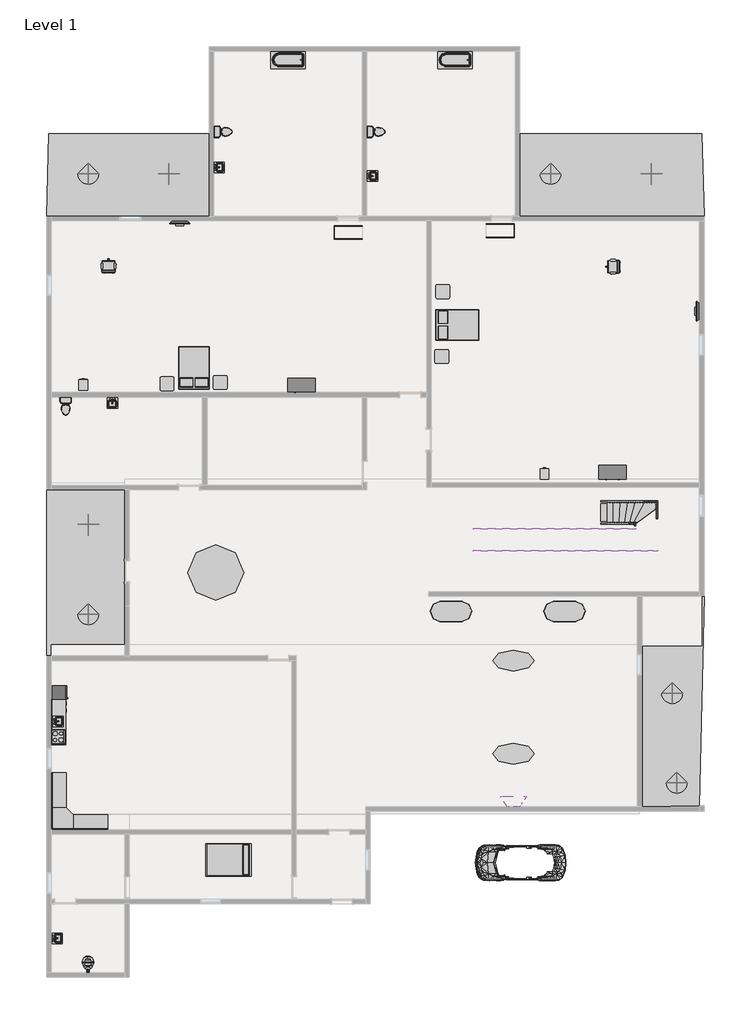
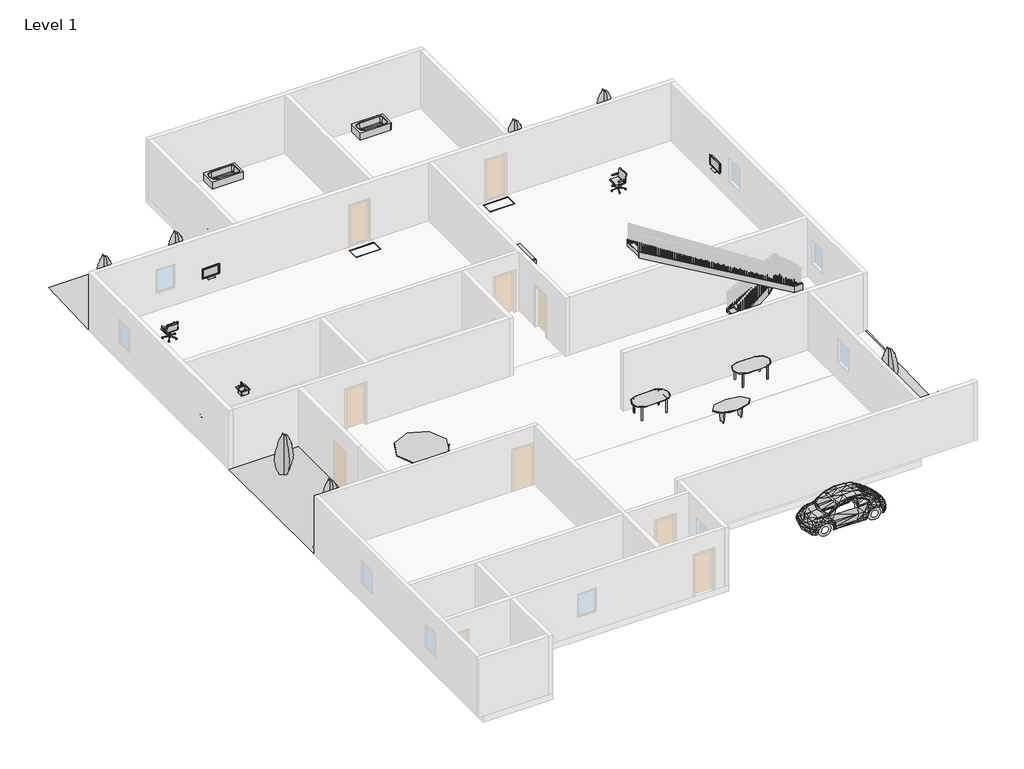
# One storey, part 4 of 4: 23 furniture elements, 11 flow terminals, 11 proxies, 8 geographic elements, 8 members, 1 stair flight.
"""IFC4 building model written with IfcOpenShell, lengths in millimetres."""

from ifc_helpers import new_model, si_unit, frame, origin, place, context, project, spatial, polyline, outline, extrude, triangles, transform, mapped, element, save
from components import proxy_a6faaae8, proxy_45b28599, kitchenette_medium_kitchenette_medium_844211aa, rpc_beetle_rpc_beetle_3ce7ba48, proxy_c523a7b7, walk_off_mat_walk_off_mat_25c2b8c1, flow_terminal_871c2e40, flow_terminal_bd37145e, toilet_domestic_3d_toilet_domestic_3d_f7549cf7, toilet_domestic_3d_toilet_domestic_3d_183bbd19, tub_rectangular_3d_tub_rectangular_3d_ca47631e, furniture_c8abb964, furniture_096e7f55, furniture_552c1472, chair_task_arms_chair_task_arms_fa5a08ef, furniture_c6510c7c, furniture_9fa109b2, furniture_56245f3a, tv_stand_tv_stand_6ce107e5, furniture_2c34a4f9, furniture_5d3b8c6f, furniture_027a2ad9, furniture_bcf351fa, furniture_45e3acac, rpc_tree_conifer_chinese_juniper_7_1b9786cd, stair_flight_225c1673

model = new_model("IFC4")

# Units and contexts
model_context = context("Model", 3, world=origin())
ifc_project = project(units=[si_unit("LENGTHUNIT", "METRE", prefix="MILLI")], contexts=[model_context])

# Site, building, storey
site = spatial("IfcSite", under=ifc_project)
building = spatial("IfcBuilding", under=site)
storey = spatial("IfcBuildingStorey", under=building, Name="Level 1", Elevation=0.0)

# Proxies
placement = place(None, origin())
element("IfcBuildingElementProxy", 1, Name="Building Element Proxy", at=placement, inside=storey, context=model_context, shape_type="Tessellation", body=[
    triangles([(-12619.2832214, 17120.266626, 0.0), (-5481.8828339, 17120.266626, 0.0), (-5583.4830276, 13500.766626, 0.0), (-12720.8828339, 13500.766626, 0.0)], [[1, 4, 3], [3, 2, 1]], closed=False),
])
element("IfcBuildingElementProxy", 2, Name="Building Element Proxy", at=placement, inside=storey, context=model_context, shape_type="Tessellation", body=[
    triangles([(7929.3171661, 17120.266626, 0.0), (16006.5171661, 17120.266626, 0.0), (16108.1167786, 13500.766626, 0.0), (8030.9173599, 13500.766626, 0.0)], [[1, 4, 2], [3, 2, 4]], closed=False),
])
element("IfcBuildingElementProxy", 3, Name="Building Element Proxy", at=placement, inside=storey, context=model_context, shape_type="Tessellation", body=[
    triangles([(-12720.8828339, 1511.9665775, 0.0), (-9291.8828339, 1511.9665775, 0.0), (-9291.8828339, -5777.833374, 0.0), (-12720.8828339, -5777.833374, 0.0)], [[1, 4, 2], [3, 2, 4]], closed=False),
])
element("IfcBuildingElementProxy", 4, Name="Building Element Proxy", at=placement, inside=storey, context=model_context, shape_type="Tessellation", body=[
    triangles([(13390.3175537, -3161.6334709, 0.0), (16108.1167786, -3161.6334709, 0.0), (13390.3175537, -12381.8337616, 0.0), (15904.9175537, -12356.4329865, 0.0)], [[1, 3, 4], [4, 2, 1]], closed=False),
])
proxy_shape = proxy_a6faaae8(model_context)
element("IfcBuildingElementProxy", 5, Name="Cook Top-4 Unit2 : 22\" x 20\"", ObjectType="Cook Top-4 Unit2 : 22\" x 20\"", at=placement, inside=storey, context=model_context, shape_type="MappedRepresentation", body=[
    mapped(proxy_shape, transform((-12212.8828173, -9321.1334604, 0.0), x_axis=(0.0, 1.0, 0.0), y_axis=(-1.0, 0.0, 0.0), z_axis=(0.0, 0.0, 1.0))),
])
proxy_2_shape = proxy_45b28599(model_context)
element("IfcBuildingElementProxy", 6, Name="Dishwasher : 24\" x 24\" x 34\"", ObjectType="Dishwasher : 24\" x 24\" x 34\"", at=placement, inside=storey, context=model_context, shape_type="MappedRepresentation", body=[
    mapped(proxy_2_shape, transform((-11921.0332525, -8369.9509289, 0.0), x_axis=(0.0, 1.0, 0.0), y_axis=(-1.0, 0.0, 0.0), z_axis=(0.0, 0.0, 1.0))),
])
kitchenette_medium_kitchenette_medium_shape = kitchenette_medium_kitchenette_medium_844211aa(model_context)
element("IfcBuildingElementProxy", 7, Name="Kitchenette - Medium : Kitchenette - Medium", ObjectType="Kitchenette - Medium : Kitchenette - Medium", at=placement, inside=storey, context=model_context, shape_type="MappedRepresentation", body=[
    mapped(kitchenette_medium_kitchenette_medium_shape, transform((-12517.6828173, -8996.9711653, 0.0), x_axis=(0.0, 1.0, 0.0), y_axis=(-1.0, 0.0, 0.0), z_axis=(0.0, 0.0, 1.0))),
])
rpc_beetle_rpc_beetle_shape = rpc_beetle_rpc_beetle_3ce7ba48(model_context)
element("IfcBuildingElementProxy", 8, Name="RPC Beetle : RPC Beetle", ObjectType="RPC Beetle : RPC Beetle", at=placement, inside=storey, context=model_context, shape_type="MappedRepresentation", body=[
    mapped(rpc_beetle_rpc_beetle_shape, transform((9300.9171827, -14845.6334604, 0.0), x_axis=(0.0, 1.0, 0.0), y_axis=(-1.0, 0.0, 0.0), z_axis=(0.0, 0.0, 1.0))),
])
proxy_3_shape = proxy_c523a7b7(model_context)
element("IfcBuildingElementProxy", 9, Name="Refrigerator : 24\" x 25\" LH", ObjectType="Refrigerator : 24\" x 25\" LH", at=placement, inside=storey, context=model_context, shape_type="MappedRepresentation", body=[
    mapped(proxy_3_shape, transform((-12167.2338458, -7384.3834604, 0.0), x_axis=(0.0, 1.0, 0.0), y_axis=(-1.0, 0.0, 0.0), z_axis=(0.0, 0.0, 1.0))),
])
walk_off_mat_walk_off_mat_shape = walk_off_mat_walk_off_mat_25c2b8c1(model_context)
element("IfcBuildingElementProxy", 10, Name="Walk-Off Mat : Walk-Off Mat", ObjectType="Walk-Off Mat : Walk-Off Mat", at=placement, inside=storey, context=model_context, shape_type="MappedRepresentation", body=[
    mapped(walk_off_mat_walk_off_mat_shape, transform((905.9526444, 13538.8606067, 0.0), x_axis=(1.0, 0.0, 0.0), y_axis=(0.0, 1.0, 0.0), z_axis=(0.0, 0.0, 1.0))),
])
element("IfcBuildingElementProxy", 11, Name="Walk-Off Mat : Walk-Off Mat", ObjectType="Walk-Off Mat : Walk-Off Mat", at=placement, inside=storey, context=model_context, shape_type="MappedRepresentation", body=[
    mapped(walk_off_mat_walk_off_mat_shape, transform((7560.7526444, 13615.0606067, 0.0), x_axis=(1.0, 0.0, 0.0), y_axis=(0.0, 1.0, 0.0), z_axis=(0.0, 0.0, 1.0))),
])

# Flow terminals
flow_terminal_shape = flow_terminal_871c2e40(model_context)
element("IfcFlowTerminal", 12, ObjectType="Sink Kitchen-Island : 18\" x 18\"", at=placement, inside=storey, context=model_context, shape_type="MappedRepresentation", body=[
    mapped(flow_terminal_shape, transform((-5162.0374161, 15631.3772991, 0.0), x_axis=(0.0, 1.0000000000000002, 0.0), y_axis=(-1.0000000000000002, 0.0, 0.0), z_axis=(0.0, 0.0, 1.0))),
])
element("IfcFlowTerminal", 13, ObjectType="Sink Kitchen-Island : 18\" x 18\"", at=placement, inside=storey, context=model_context, shape_type="MappedRepresentation", body=[
    mapped(flow_terminal_shape, transform((1568.9625839, 15250.3772991, 0.0), x_axis=(0.0, 1.0000000000000009, 0.0), y_axis=(-1.0000000000000009, 0.0, 0.0), z_axis=(0.0, 0.0, 1.0))),
])
element("IfcFlowTerminal", 14, ObjectType="Sink Kitchen-Island : 18\" x 18\"", at=placement, inside=storey, context=model_context, shape_type="MappedRepresentation", body=[
    mapped(flow_terminal_shape, transform((-9853.6720578, 5306.9211385, 0.0), x_axis=(1.0, 0.0, 0.0), y_axis=(0.0, 1.0, 0.0), z_axis=(0.0, 0.0, 1.0))),
])
element("IfcFlowTerminal", 15, ObjectType="Sink Kitchen-Island : 18\" x 18\"", at=placement, inside=storey, context=model_context, shape_type="MappedRepresentation", body=[
    mapped(flow_terminal_shape, transform((-12210.5374161, -8663.7227009, -14.4), x_axis=(0.0, 1.0, 0.0), y_axis=(-1.0, 0.0, 0.0), z_axis=(0.0, 0.0, 1.0))),
])
element("IfcFlowTerminal", 16, ObjectType="Sink Kitchen-Island : 18\" x 18\"", at=placement, inside=storey, context=model_context, shape_type="MappedRepresentation", body=[
    mapped(flow_terminal_shape, transform((-12248.6374161, -18176.0227009, 0.0), x_axis=(0.0, 1.0000000000000002, 0.0), y_axis=(-1.0000000000000002, 0.0, 0.0), z_axis=(0.0, 0.0, 1.0))),
])
flow_terminal_2_shape = flow_terminal_bd37145e(model_context)
element("IfcFlowTerminal", 17, ObjectType="Toilet-Commercial-Wall-3D : 15\" Seat Height", at=placement, inside=storey, context=model_context, shape_type="MappedRepresentation", body=[
    mapped(flow_terminal_2_shape, transform((-11309.6859711, -19773.2334604, 0.0), x_axis=(1.0, 0.0, 0.0), y_axis=(0.0, 1.0, 0.0), z_axis=(0.0, 0.0, 1.0))),
])
toilet_domestic_3d_toilet_domestic_3d_shape = toilet_domestic_3d_toilet_domestic_3d_f7549cf7(model_context)
toilet_domestic_3d_toilet_domestic_3d_2_shape = toilet_domestic_3d_toilet_domestic_3d_183bbd19(model_context)
element("IfcFlowTerminal", 18, ObjectType="Toilet-Domestic-3D : Toilet-Domestic-3D", at=placement, inside=storey, context=model_context, shape_type="MappedRepresentation", body=[
    mapped(toilet_domestic_3d_toilet_domestic_3d_shape, transform((-4885.5867899, 17203.8414884, 0.0), x_axis=(0.0, 1.0000000000000002, 0.0), y_axis=(-1.0000000000000002, 0.0, 0.0), z_axis=(0.0, 0.0, 1.0))),
    mapped(toilet_domestic_3d_toilet_domestic_3d_2_shape, transform((-4885.5867899, 17203.8414884, 0.0), x_axis=(0.0, 1.0000000000000002, 0.0), y_axis=(-1.0000000000000002, 0.0, 0.0), z_axis=(0.0, 0.0, 1.0))),
])
element("IfcFlowTerminal", 19, ObjectType="Toilet-Domestic-3D : Toilet-Domestic-3D", at=placement, inside=storey, context=model_context, shape_type="MappedRepresentation", body=[
    mapped(toilet_domestic_3d_toilet_domestic_3d_shape, transform((1820.0132101, 17203.8414884, 0.0), x_axis=(0.0, 1.0000000000000002, 0.0), y_axis=(-1.0000000000000002, 0.0, 0.0), z_axis=(0.0, 0.0, 1.0))),
    mapped(toilet_domestic_3d_toilet_domestic_3d_2_shape, transform((1820.0132101, 17203.8414884, 0.0), x_axis=(0.0, 1.0000000000000002, 0.0), y_axis=(-1.0000000000000002, 0.0, 0.0), z_axis=(0.0, 0.0, 1.0))),
])
element("IfcFlowTerminal", 20, ObjectType="Toilet-Domestic-3D : Toilet-Domestic-3D", at=placement, inside=storey, context=model_context, shape_type="MappedRepresentation", body=[
    mapped(toilet_domestic_3d_toilet_domestic_3d_shape, transform((-11882.6828173, 5081.2705123, 0.0), x_axis=(1.0, 0.0, 0.0), y_axis=(0.0, 1.0, 0.0), z_axis=(0.0, 0.0, 1.0))),
    mapped(toilet_domestic_3d_toilet_domestic_3d_2_shape, transform((-11882.6828173, 5081.2705123, 0.0), x_axis=(1.0, 0.0, 0.0), y_axis=(0.0, 1.0, 0.0), z_axis=(0.0, 0.0, 1.0))),
])
tub_rectangular_3d_tub_rectangular_3d_shape = tub_rectangular_3d_tub_rectangular_3d_ca47631e(model_context)
element("IfcFlowTerminal", 21, ObjectType="Tub-Rectangular-3D : Tub-Rectangular-3D", at=placement, inside=storey, context=model_context, shape_type="MappedRepresentation", body=[
    mapped(tub_rectangular_3d_tub_rectangular_3d_shape, transform((-2477.685786, 20841.3665396, 0.0), x_axis=(-1.0, 0.0, 0.0), y_axis=(0.0, -1.0, 0.0), z_axis=(0.0, 0.0, 1.0))),
])
element("IfcFlowTerminal", 22, ObjectType="Tub-Rectangular-3D : Tub-Rectangular-3D", at=placement, inside=storey, context=model_context, shape_type="MappedRepresentation", body=[
    mapped(tub_rectangular_3d_tub_rectangular_3d_shape, transform((4837.514214, 20841.3665396, 0.0), x_axis=(-1.0, 0.0, 0.0), y_axis=(0.0, -1.0, 0.0), z_axis=(0.0, 0.0, 1.0))),
])

# Furniture
furniture_shape = furniture_c8abb964(model_context)
element("IfcFurniture", 23, ObjectType="Bed-Box : Double 53\" x 74\"", at=placement, inside=storey, context=model_context, shape_type="MappedRepresentation", body=[
    mapped(furniture_shape, transform((-5917.4303582, 6611.5370314, 0.0), x_axis=(-1.0000000000000002, 0.0, 0.0), y_axis=(0.0, -1.0000000000000002, 0.0), z_axis=(0.0, 0.0, 1.0))),
])
element("IfcFurniture", 24, ObjectType="Bed-Box : Double 53\" x 74\"", at=placement, inside=storey, context=model_context, shape_type="MappedRepresentation", body=[
    mapped(furniture_shape, transform((5053.2876745, 8399.1140806, 0.0), x_axis=(0.0, 1.0000000000000002, 0.0), y_axis=(-1.0000000000000002, 0.0, 0.0), z_axis=(0.0, 0.0, 1.0))),
])
furniture_2_shape = furniture_096e7f55(model_context)
element("IfcFurniture", 25, ObjectType="Bed-Shaker : Double 56\" x 78\"", at=placement, inside=storey, context=model_context, shape_type="MappedRepresentation", body=[
    mapped(furniture_2_shape, transform((-3754.6828173, -14737.6834604, 0.0), x_axis=(0.0, -1.0000000000000002, 0.0), y_axis=(1.0000000000000002, 0.0, 0.0), z_axis=(0.0, 0.0, 1.0))),
])
furniture_3_shape = furniture_552c1472(model_context)
element("IfcFurniture", 26, ObjectType="Cabinet-File 3 Drawer : 15\" x 18\"", at=placement, inside=storey, context=model_context, shape_type="MappedRepresentation", body=[
    mapped(furniture_3_shape, transform((-11235.8792643, 5967.2322395, 0.0), x_axis=(-1.0000000000000004, 0.0, 0.0), y_axis=(0.0, -1.0000000000000004, 0.0), z_axis=(0.0, 0.0, 1.0))),
])
element("IfcFurniture", 27, ObjectType="Cabinet-File 3 Drawer : 15\" x 18\"", at=placement, inside=storey, context=model_context, shape_type="MappedRepresentation", body=[
    mapped(furniture_3_shape, transform((8982.5207357, 2055.6322395, 0.0), x_axis=(-1.0000000000000004, 0.0, 0.0), y_axis=(0.0, -1.0000000000000004, 0.0), z_axis=(0.0, 0.0, 1.0))),
])
chair_task_arms_chair_task_arms_shape = chair_task_arms_chair_task_arms_fa5a08ef(model_context)
element("IfcFurniture", 28, ObjectType="Chair-Task Arms : Chair-Task Arms", at=placement, inside=storey, context=model_context, shape_type="MappedRepresentation", body=[
    mapped(chair_task_arms_chair_task_arms_shape, transform((-10144.0736369, 11272.020638, 0.0), x_axis=(1.0, 0.0, 0.0), y_axis=(0.0, 1.0, 0.0), z_axis=(0.0, 0.0, 1.0))),
])
element("IfcFurniture", 29, ObjectType="Chair-Task Arms : Chair-Task Arms", at=placement, inside=storey, context=model_context, shape_type="MappedRepresentation", body=[
    mapped(chair_task_arms_chair_task_arms_shape, transform((12164.6630844, 11149.97572, 0.0), x_axis=(0.0, 1.0000000000000002, 0.0), y_axis=(-1.0000000000000002, 0.0, 0.0), z_axis=(0.0, 0.0, 1.0))),
])
furniture_4_shape = furniture_c6510c7c(model_context)
element("IfcFurniture", 30, ObjectType="Counter Top w Sink Hole : 24\" Depth", at=placement, inside=storey, context=model_context, shape_type="MappedRepresentation", body=[
    mapped(furniture_4_shape, transform((-12517.6828173, -8463.5711653, -14.4), x_axis=(0.0, 1.0, 0.0), y_axis=(-1.0, 0.0, 0.0), z_axis=(0.0, 0.0, 1.0))),
])
furniture_5_shape = furniture_9fa109b2(model_context)
element("IfcFurniture", 31, ObjectType="Dresser : 48\" x 72\" x 24\"", at=placement, inside=storey, context=model_context, shape_type="MappedRepresentation", body=[
    mapped(furniture_5_shape, transform((12364.1104426, 2637.1294937, 0.0), x_axis=(1.0, 0.0, 0.0), y_axis=(0.0, 1.0, 0.0), z_axis=(0.0, 0.0, 1.0))),
])
element("IfcFurniture", 32, ObjectType="Dresser : 48\" x 72\" x 24\"", at=placement, inside=storey, context=model_context, shape_type="MappedRepresentation", body=[
    mapped(furniture_5_shape, transform((-1275.6895574, 6447.1294937, 0.0), x_axis=(1.0, 0.0, 0.0), y_axis=(0.0, 1.0, 0.0), z_axis=(0.0, 0.0, 1.0))),
])
furniture_6_shape = furniture_56245f3a(model_context)
element("IfcFurniture", 33, ObjectType="TV - Flat Screen : 32\"", at=placement, inside=storey, context=model_context, shape_type="MappedRepresentation", body=[
    mapped(furniture_6_shape, transform((-6874.9383031, 13239.027916, 914.4), x_axis=(1.0, 0.0, 0.0), y_axis=(0.0, 1.0, 0.0), z_axis=(0.0, 0.0, 1.0))),
])
element("IfcFurniture", 34, ObjectType="TV - Flat Screen : 32\"", at=placement, inside=storey, context=model_context, shape_type="MappedRepresentation", body=[
    mapped(furniture_6_shape, transform((15846.3785591, 9331.2220255, 914.4), x_axis=(0.0, -1.0000000000000002, 0.0), y_axis=(1.0000000000000002, 0.0, 0.0), z_axis=(0.0, 0.0, 1.0))),
])
tv_stand_tv_stand_shape = tv_stand_tv_stand_6ce107e5(model_context)
element("IfcFurniture", 35, ObjectType="TV Stand : TV Stand", at=placement, inside=storey, context=model_context, shape_type="MappedRepresentation", body=[
    mapped(tv_stand_tv_stand_shape, transform((7876.7051848, -12381.8334604, 1219.2), x_axis=(-1.0000000000000002, 0.0, 0.0), y_axis=(0.0, -1.0000000000000002, 0.0), z_axis=(0.0, 0.0, 1.0))),
])
furniture_7_shape = furniture_2c34a4f9(model_context)
element("IfcFurniture", 36, ObjectType="Table-Dining Oval : 36\" x 72\"", at=placement, inside=storey, context=model_context, shape_type="MappedRepresentation", body=[
    mapped(furniture_7_shape, transform((5410.1368549, -3470.2850997, 0.0), x_axis=(1.0, 0.0, 0.0), y_axis=(0.0, 1.0, 0.0), z_axis=(0.0, 0.0, 1.0))),
])
element("IfcFurniture", 37, ObjectType="Table-Dining Oval : 36\" x 72\"", at=placement, inside=storey, context=model_context, shape_type="MappedRepresentation", body=[
    mapped(furniture_7_shape, transform((10388.5368549, -3470.2850997, 0.0), x_axis=(1.0, 0.0, 0.0), y_axis=(0.0, 1.0, 0.0), z_axis=(0.0, 0.0, 1.0))),
])
furniture_8_shape = furniture_5d3b8c6f(model_context)
element("IfcFurniture", 38, ObjectType="Table-Dining Round w Chairs : 84\" Diameter", at=placement, inside=storey, context=model_context, shape_type="MappedRepresentation", body=[
    mapped(furniture_8_shape, transform((-5407.7647845, -1935.3547718, 0.0), x_axis=(1.0, 0.0, 0.0), y_axis=(0.0, 1.0, 0.0), z_axis=(0.0, 0.0, 1.0))),
])
furniture_9_shape = furniture_027a2ad9(model_context)
element("IfcFurniture", 39, ObjectType="Table-Ellipse : 72\" x 36\"", at=placement, inside=storey, context=model_context, shape_type="MappedRepresentation", body=[
    mapped(furniture_9_shape, transform((7751.5171827, -5981.0334604, 0.0), x_axis=(1.0, 0.0, 0.0), y_axis=(0.0, 1.0, 0.0), z_axis=(0.0, 0.0, 1.0))),
])
element("IfcFurniture", 40, ObjectType="Table-Ellipse : 72\" x 36\"", at=placement, inside=storey, context=model_context, shape_type="MappedRepresentation", body=[
    mapped(furniture_9_shape, transform((7751.5171827, -10070.4334604, 0.0), x_axis=(1.0, 0.0, 0.0), y_axis=(0.0, 1.0, 0.0), z_axis=(0.0, 0.0, 1.0))),
])
furniture_10_shape = furniture_bcf351fa(model_context)
element("IfcFurniture", 41, ObjectType="Table-End : 24\" x 24\"", at=placement, inside=storey, context=model_context, shape_type="MappedRepresentation", body=[
    mapped(furniture_10_shape, transform((-5409.4164475, 6058.5665396, 0.0), x_axis=(1.0, 0.0, 0.0), y_axis=(0.0, 1.0, 0.0), z_axis=(0.0, 0.0, 1.0))),
])
element("IfcFurniture", 42, ObjectType="Table-End : 24\" x 24\"", at=placement, inside=storey, context=model_context, shape_type="MappedRepresentation", body=[
    mapped(furniture_10_shape, transform((-7746.2164475, 6007.7665396, 0.0), x_axis=(1.0, 0.0, 0.0), y_axis=(0.0, 1.0, 0.0), z_axis=(0.0, 0.0, 1.0))),
])
element("IfcFurniture", 43, ObjectType="Table-End : 24\" x 24\"", at=placement, inside=storey, context=model_context, shape_type="MappedRepresentation", body=[
    mapped(furniture_10_shape, transform((4293.3835525, 7201.5665396, 0.0), x_axis=(1.0, 0.0, 0.0), y_axis=(0.0, 1.0, 0.0), z_axis=(0.0, 0.0, 1.0))),
])
element("IfcFurniture", 44, ObjectType="Table-End : 24\" x 24\"", at=placement, inside=storey, context=model_context, shape_type="MappedRepresentation", body=[
    mapped(furniture_10_shape, transform((4805.1171827, 9890.2329094, 0.0), x_axis=(0.0, 1.0, 0.0), y_axis=(-1.0, 0.0, 0.0), z_axis=(0.0, 0.0, 1.0))),
])
furniture_11_shape = furniture_45e3acac(model_context)
element("IfcFurniture", 45, ObjectType="Work Station Cubicle : 96\" x 96\"", at=placement, inside=storey, context=model_context, shape_type="MappedRepresentation", body=[
    mapped(furniture_11_shape, transform((-13012.7058249, -13266.1017081, 0.0), x_axis=(0.0, 1.0000000000000002, 0.0), y_axis=(-1.0000000000000002, 0.0, 0.0), z_axis=(0.0, 0.0, 1.0))),
])

# Geographic elements
rpc_tree_conifer_chinese_juniper_7_shape = rpc_tree_conifer_chinese_juniper_7_1b9786cd(model_context)
element("IfcGeographicElement", 46, ObjectType="RPC Tree - Conifer : Chinese Juniper - 7'", at=placement, inside=storey, context=model_context, shape_type="MappedRepresentation", body=[
    mapped(rpc_tree_conifer_chinese_juniper_7_shape, transform((14710.9205117, -7403.4334604, 0.0), x_axis=(1.0, 0.0, 0.0), y_axis=(0.0, 1.0, 0.0), z_axis=(0.0, 0.0, 1.0))),
])
element("IfcGeographicElement", 47, ObjectType="RPC Tree - Conifer : Chinese Juniper - 7'", at=placement, inside=storey, context=model_context, shape_type="MappedRepresentation", body=[
    mapped(rpc_tree_conifer_chinese_juniper_7_shape, transform((14914.1205117, -11340.4334604, 0.0), x_axis=(1.0, 0.0, 0.0), y_axis=(0.0, 1.0, 0.0), z_axis=(0.0, 0.0, 1.0))),
])
element("IfcGeographicElement", 48, ObjectType="RPC Tree - Conifer : Chinese Juniper - 7'", at=placement, inside=storey, context=model_context, shape_type="MappedRepresentation", body=[
    mapped(rpc_tree_conifer_chinese_juniper_7_shape, transform((-10892.2794883, -12.0334604, 0.0), x_axis=(1.0, 0.0, 0.0), y_axis=(0.0, 1.0, 0.0), z_axis=(0.0, 0.0, 1.0))),
])
element("IfcGeographicElement", 49, ObjectType="RPC Tree - Conifer : Chinese Juniper - 7'", at=placement, inside=storey, context=model_context, shape_type="MappedRepresentation", body=[
    mapped(rpc_tree_conifer_chinese_juniper_7_shape, transform((-10892.2794883, -3949.0334604, 0.0), x_axis=(1.0, 0.0, 0.0), y_axis=(0.0, 1.0, 0.0), z_axis=(0.0, 0.0, 1.0))),
])
element("IfcGeographicElement", 50, ObjectType="RPC Tree - Conifer : Chinese Juniper - 7'", at=placement, inside=storey, context=model_context, shape_type="MappedRepresentation", body=[
    mapped(rpc_tree_conifer_chinese_juniper_7_shape, transform((-10892.2794883, 15367.6665396, 0.0), x_axis=(1.0, 0.0, 0.0), y_axis=(0.0, 1.0, 0.0), z_axis=(0.0, 0.0, 1.0))),
])
element("IfcGeographicElement", 51, ObjectType="RPC Tree - Conifer : Chinese Juniper - 7'", at=placement, inside=storey, context=model_context, shape_type="MappedRepresentation", body=[
    mapped(rpc_tree_conifer_chinese_juniper_7_shape, transform((-7361.6794883, 15367.6665396, 0.0), x_axis=(1.0, 0.0, 0.0), y_axis=(0.0, 1.0, 0.0), z_axis=(0.0, 0.0, 1.0))),
])
element("IfcGeographicElement", 52, ObjectType="RPC Tree - Conifer : Chinese Juniper - 7'", at=placement, inside=storey, context=model_context, shape_type="MappedRepresentation", body=[
    mapped(rpc_tree_conifer_chinese_juniper_7_shape, transform((9376.9205117, 15367.6665396, 0.0), x_axis=(1.0, 0.0, 0.0), y_axis=(0.0, 1.0, 0.0), z_axis=(0.0, 0.0, 1.0))),
])
element("IfcGeographicElement", 53, ObjectType="RPC Tree - Conifer : Chinese Juniper - 7'", at=placement, inside=storey, context=model_context, shape_type="MappedRepresentation", body=[
    mapped(rpc_tree_conifer_chinese_juniper_7_shape, transform((13796.5205117, 15367.6665396, 0.0), x_axis=(1.0, 0.0, 0.0), y_axis=(0.0, 1.0, 0.0), z_axis=(0.0, 0.0, 1.0))),
])

# Members
element("IfcMember", 54, ObjectType="Stringer - 2\" Width", at=placement, inside=storey, context=model_context, shape_type="SweptSolid", body=[
    extrude(outline(polyline([(229.639954, 11576.2992414), (0.0, 11576.2992414), (0.0, 11796.0615589), (962.500629, 13663.7164331), (1305.3956453, 13663.7164331), (229.639954, 11576.2992414)])), frame((0.0, 971.4275916, 0.0), z_axis=(0.0, 1.0, 0.0), x_axis=(0.0, 0.0, 1.0)), (0.0, 0.0, 1.0), 50.8),
])
element("IfcMember", 55, ObjectType="Stringer - 2\" Width", at=placement, inside=storey, context=model_context, shape_type="SweptSolid", body=[
    extrude(outline(polyline([(13663.7164331, 971.4275916), (13663.7164331, 1022.2275916), (14018.4309332, 1022.2275916), (14018.4309332, 971.4275916), (13663.7164331, 971.4275916)])), frame((0.0, 0.0, 962.500629), z_axis=(0.0, 0.0, 1.0), x_axis=(1.0, 0.0, 0.0)), (0.0, 0.0, 1.0), 342.8950162),
])
element("IfcMember", 56, ObjectType="Stringer - 2\" Width", at=placement, inside=storey, context=model_context, shape_type="SweptSolid", body=[
    extrude(outline(polyline([(1022.2275916, 1289.0952212), (1022.2275916, 1000.5956453), (852.7051086, 1000.5956453), (-1136.7724084, 1638.9682298), (-1136.7724084, 1969.9972697), (-1099.7922911, 1969.9972697), (1022.2275916, 1289.0952212)])), frame((14018.4309332, 0.0, 0.0), z_axis=(1.0, 0.0, 0.0), x_axis=(0.0, 1.0, 0.0)), (0.0, 0.0, 1.0), 50.8),
])
element("IfcMember", 57, ObjectType="Stringer - 2\" Width", at=placement, inside=storey, context=model_context, shape_type="SweptSolid", body=[
    extrude(outline(polyline([(14069.2309332, -1136.7724084), (14069.2309332, -1187.5724084), (13643.9447902, -1187.5724084), (13643.9447902, -1136.7724084), (14069.2309332, -1136.7724084)])), frame((0.0, 0.0, 1649.8904473), z_axis=(0.0, 0.0, 1.0), x_axis=(1.0, 0.0, 0.0)), (0.0, 0.0, 1.0), 320.1068224),
])
element("IfcMember", 58, ObjectType="Stringer - 2\" Width", at=placement, inside=storey, context=model_context, shape_type="SweptSolid", body=[
    extrude(outline(polyline([(1649.8904473, 13643.9447902), (1969.9972697, 13643.9447902), (6452.0052414, 5988.2992414), (6131.898419, 5988.2992414), (1649.8904473, 13643.9447902)])), frame((0.0, -1187.5724084, 0.0), z_axis=(0.0, 1.0, 0.0), x_axis=(0.0, 0.0, 1.0)), (0.0, 0.0, 1.0), 50.8),
])
element("IfcMember", 59, ObjectType="Stringer - 2\" Width", at=placement, inside=storey, context=model_context, shape_type="SweptSolid", body=[
    extrude(outline(polyline([(176.1764461, 11576.2992414), (0.0, 11576.2992414), (0.0, 11842.5608859), (987.1410923, 13053.2309332), (1380.418648, 13053.2309332), (176.1764461, 11576.2992414)])), frame((0.0, 6.2275916, 0.0), z_axis=(0.0, 1.0, 0.0), x_axis=(0.0, 0.0, 1.0)), (0.0, 0.0, 1.0), 50.8),
])
element("IfcMember", 60, ObjectType="Stringer - 2\" Width", at=placement, inside=storey, context=model_context, shape_type="SweptSolid", body=[
    extrude(outline(polyline([(57.0275916, 1573.2682978), (57.0275916, 1028.5617647), (22.7853743, 1028.5617647), (-171.5724084, 1360.465107), (-171.5724084, 1907.6561096), (-138.7850604, 1907.6561096), (57.0275916, 1573.2682978)])), frame((13053.2309332, 0.0, 0.0), z_axis=(1.0, 0.0, 0.0), x_axis=(0.0, 1.0, 0.0)), (0.0, 0.0, 1.0), 50.8),
])
element("IfcMember", 61, ObjectType="Stringer - 2\" Width", at=placement, inside=storey, context=model_context, shape_type="SweptSolid", body=[
    extrude(outline(polyline([(1545.0818941, 13104.0309332), (1907.6561096, 13104.0309332), (6491.7799492, 5988.2992414), (6129.2057337, 5988.2992414), (1545.0818941, 13104.0309332)])), frame((0.0, -222.3724084, 0.0), z_axis=(0.0, 1.0, 0.0), x_axis=(0.0, 0.0, 1.0)), (0.0, 0.0, 1.0), 50.8),
])

# Stair flight
stair_flight_shape = stair_flight_225c1673(model_context)
element("IfcStairFlight", 62, ObjectType="2\" Tread 1\" Nosing 1/4\" Riser", at=placement, inside=storey, context=model_context, shape_type="MappedRepresentation", body=[
    mapped(stair_flight_shape, transform((0.0, 0.0, 0.0), x_axis=(1.0, 0.0, 0.0), y_axis=(0.0, 1.0, 0.0), z_axis=(0.0, 0.0, 1.0))),
])

save(model, "model.ifc")

# Revit data of these elements
# Type "Cook Top-4 Unit2 : 22\" x 20\""
#   Depth = 1' - 8"
#   Width = 1' - 10"
#   Burner Material = Steel, Chrome Plated
#   Cooktop Material = Steel, Polished
#   Default Elevation = 0
#   Assembly Code = ""
# Type "Dishwasher : 24\" x 24\" x 34\""
#   Label = "DW"
#   Assembly Code = "E1090400"
#   Depth = 2' - 0"
#   Height = 2' - 10"
#   Width = 2' - 0"
#   Dishwasher Material = Steel, Paint Finish, Ivory, Glossy
#   Panel Face Material = Plastic, Opaque Black
#   Default Elevation = 0
# Type "Kitchenette - Medium : Kitchenette - Medium"
#   Assembly Code = "E1090400"
#   Counter Length = 6' - 6"
#   Cabinet Width = 4' - 6"
#   Cabinet Height = 2' - 10 1/2"
#   Cabinet Depth = 2' - 0"
#   Toe Depth = 0' - 3"
#   Toe Height = 0' - 3 1/2"
#   Cabinet Material = Cabinets
#   Door/Drawer Material = Cabinets
#   Handle Material = Cabinets - Handles
#   Default Elevation = 0
# Type "RPC Beetle : RPC Beetle"
#   built-in parameter 1005195 = "RPC-16-0U6E-L4EG-ENH1-J3KF-SVEL-0TX4-C0"
#   Height = 0
# Type "Refrigerator : 24\" x 25\" LH"
#   Label = "REF."
#   Assembly Code = "E1090400"
#   Depth = 2' - 0 3/4"
#   Handle = 0' - 1 1/2"
#   Height = 5' - 3 1/2"
#   Rear Clearance = 0' - 2"
#   Top Door Height = 1' - 8"
#   Width = 1' - 11 1/2"
#   Material = Steel, Paint Finish, Ivory, Glossy
#   Default Elevation = 0
# Type "Walk-Off Mat : Walk-Off Mat"
#   Width [instance default] = 4' - 0"
#   Length [instance default] = 2' - 0"
#   Array Length [instance default] = 1' - 10"
#   WebArrayNum [instance default] = 18
#   Default Elevation = 0
# Type "Sink Kitchen-Island : 18\" x 18\""
#   Assembly Code = "D2010410"
#   Counter Height = 3' - 0"
#   Depth = 1' - 6"
#   Width = 1' - 6"
#   Faucet Material = Steel, Polished
#   Sink Material = Steel, Polished
#   Default Elevation = 0
# Type "Toilet-Commercial-Wall-3D : 15\" Seat Height"
#   Assembly Code = "D2010110"
#   Mounting Height = 1' - 3"
#   Piping Material = Steel, Polished
#   Toilet - Bowl Material = Porcelain, Ivory
#   Toilet - Seat Material = Laminate, Ivory, Matte
#   Default Elevation = 0
# Type "Toilet-Domestic-3D : Toilet-Domestic-3D"
#   Assembly Code = "D2010110"
#   Toilet - Bowl/Basin Material = Porcelain, Linen
#   Toilet - Seat Material = Laminate, Linen, Matte
#   Default Elevation = 0
# Type "Tub-Rectangular-3D : Tub-Rectangular-3D"
#   Assembly Code = "D2010500"
#   Depth = 2' - 6"
#   Height = 1' - 3"
#   Width = 5' - 0"
#   Tub Material = Porcelain, Ivory
#   Default Elevation = 0
# Type "Bed-Box : Double 53\" x 74\""
#   Assembly Code = "E2020200"
#   Length = 6' - 2"
#   Width = 4' - 5"
#   Frame Material = Birch
#   Mattress Material = Linen, White
#   Default Elevation = 0
# Type "Bed-Shaker : Double 56\" x 78\""
#   Assembly Code = "E2020200"
#   Length = 6' - 6"
#   Width = 4' - 8"
#   Frame Material = Birch
#   Mattress Material = Linen, White
#   Default Elevation = 0
# Type "Cabinet-File 3 Drawer : 15\" x 18\""
#   Assembly Code = "E2020200"
#   Depth = 1' - 6"
#   Height = 3' - 5"
#   Width = 1' - 3"
#   Cabinet Material = Steel, Paint Finish, Ivory, Glossy
#   Handle Material = Steel, Chrome Plated
#   Default Elevation = 0
# Type "Chair-Task Arms : Chair-Task Arms"
#   Assembly Code = "E2020200"
#   Base Material = Plastic, Opaque Black
#   Caster Material = Plastic, Opaque Black
#   Seat/Back Material = Textile - Slate Blue
#   Default Elevation = 0
# Type "Counter Top w Sink Hole : 24\" Depth"
#   Assembly Code = "C1030400"
#   Counter Thickness = 0' - 1 1/2"
#   Depth = 2' - 1"
#   Height = 3' - 0"
#   Length [instance default] = 8' - 0"
#   Sink Location [instance default] = 2' - 0"
#   Sink Location To Wall [instance default] = 0' - 6"
#   Sink Opening Depth [instance default] = 1' - 3"
#   Sink Opening Width [instance default] = 2' - 3"
#   Counter Top Material = none
#   Default Elevation = 0
# Type "Dresser : 48\" x 72\" x 24\""
#   Assembly Code = "E2020200"
#   Depth = 2' - 0"
#   Height = 6' - 0"
#   Width = 4' - 0"
#   Dresser Material = Laminate - Ivory, Glossy
#   Drawer Material = Laminate, Ivory, Matte
#   Knob Material = Cherry
#   Default Elevation = 0
# Type "TV - Flat Screen : 32\""
#   SinAng = 0' - 0.0193"
#   L = 2' - 3.79372"
#   H = 1' - 3.6354"
#   Thickness = 0' - 4.33071"
#   Diagonal = 2' - 7.88976"
#   CosAng = 0' - 0.03431"
#   Stand [instance default] = yes
#   Default Elevation = 0
# Type "TV Stand : TV Stand"
#   Depth = 1' - 6"
#   Width = 3' - 8"
#   Height = 1' - 7 1/2"
#   Finish = Melamine - Gray
#   Default Elevation = 0
# Type "Table-Dining Oval : 36\" x 72\""
#   Assembly Code = "E2020200"
#   Length = 6' - 0"
#   Width = 3' - 0"
#   Base Material = Steel, Chrome Plated
#   Top Material = Glass - Clear, Grey
#   Default Elevation = 0
#   Description = (empty or 0)
# Type "Table-Dining Round w Chairs : 84\" Diameter"
#   Assembly Code = "E2020200"
#   Radius = 4' - 0"
#   Diameter = 8' - 0"
#   Height = 2' - 6"
#   Chairs = 10
#   Base Material = Pine
#   Top Material = Laminate, Linen, Matte
#   Default Elevation = 0
# Type "Table-Ellipse : 72\" x 36\""
#   Assembly Code = "E2020200"
#   Half Width = 1' - 6"
#   Half Length = 3' - 0"
#   Height = 2' - 6"
#   Length = 6' - 0"
#   Width = 3' - 0"
#   Base Material = Birch
#   Top Material = Laminate - Black
#   Default Elevation = 0
# Type "Table-End : 24\" x 24\""
#   Assembly Code = "E2020200"
#   Height = 2' - 6"
#   Length = 2' - 0"
#   Width = 2' - 0"
#   Base Material = Birch
#   Top Material = Laminate, Ivory, Matte
#   Default Elevation = 0
# Type "Work Station Cubicle : 96\" x 96\""
#   Assembly Code = "E2020"
#   Desktop Height = 2' - 6"
#   Desktop1 Width = 2' - 0"
#   Desktop2 Width = 2' - 0"
#   Panel Height = 5' - 6"
#   Panel1 Length = 5' - 0"
#   Panel2 Length = 5' - 0"
#   Cube Panel Material = Textile - Light Gray
#   Work Top Material = Laminate, Ivory, Matte
#   Default Elevation = 0
# Type "RPC Tree - Conifer : Chinese Juniper - 7'"
#   built-in parameter 1005198 = "{2, 15},{39, RPC-16-FUM3-UUQ0-UBF0-N000-ST1L-LVER-AU},{1, 0},{1, 0},{2, 13},{1, 8},{5, Color},{1, 0},{1, 0},{3, 0.8},{3, 0.8},{3, 0.8},{1, 8},{7, BBoxMin},{1, 0},{1, 0},{1, 0},{1, 0},{1, 0},{1, 8},{7, BBoxMax},{1, 0},{1, 0},{1, 0},{1, 0},{1, 0},{2, 11},{9, RPCTypeId},{1, 0},{1, 0},{39, RPC-16-FUM3-UUQ0-UBF0-N000-ST1L-LVER-AU},{1, 6},{14, RPCPlantHeight},{1, 0},{1, 0},{1, 7},{2, 11},{7, keyword},{1, 0},{1, 0},{34, :RPCs:Trees [General]:Geometry:RPC},{2, 11},{8, category},{1, 0},{1, 0},{15, Trees [General]},{2, 11},{12, LocalizedUID},{1, 0},{1, 0},{15, Chinese Juniper},{2, 14},{6, Height},{1, 0},{1, 0},{1, 7},{1, 2},{16, Cast Reflections},{1, 0},{1, 0},{1, 0},{1, 2},{12, Cast Shadows},{1, 0},{1, 0},{1, 1},{1, 2},{9, Lock View},{1, 0},{1, 0},{1, 0},{1, 4},{5, ViewC},{1, 0},{1, 0},{1, 0},{21, assetlibrary_base.fbx},{1, 5},"
#   built-in parameter 1005195 = "RPC-16-FUM3-UUQ0-UBF0-N000-ST1L-LVER-AU"
#   Type Comments = "Chinese Juniper"
#   Assembly Code = "G2050500"
#   Height = 7' - 0"
#   Description = (empty or 0)
#   Default Elevation = 0
# Elements 1, 2, 3, 4 (IfcBuildingElementProxy)
#   Material = none
#   Phase Created = New Construction
# Element 5 (IfcBuildingElementProxy, "Cook Top-4 Unit2 : 22\" x 20\"")
#   Phase Created = New Construction
#   Materials on its faces: "Steel, Chrome Plated", "Steel, Polished"
# Element 6 (IfcBuildingElementProxy, "Dishwasher : 24\" x 24\" x 34\"")
#   Phase Created = New Construction
#   Materials on its faces: "Steel, Paint Finish, Ivory, Glossy", "Plastic, Opaque Black"
# Element 7 (IfcBuildingElementProxy, "Kitchenette - Medium : Kitchenette - Medium")
#   Phase Created = New Construction
#   Materials on its faces: "Cabinets", "Cabinets - Handles"
# Element 8 (IfcBuildingElementProxy, "RPC Beetle : RPC Beetle")
#   Phase Created = New Construction
# Element 9 (IfcBuildingElementProxy, "Refrigerator : 24\" x 25\" LH")
#   Phase Created = New Construction
#   Materials on its faces: "Steel, Paint Finish, Ivory, Glossy", "Steel, Chrome Plated"
# Elements 10, 11 (IfcBuildingElementProxy, "Walk-Off Mat : Walk-Off Mat")
#   Width = 4' - 0"
#   Length = 2' - 0"
#   Array Length = 1' - 10"
#   WebArrayNum = 18
#   Phase Created = New Construction
#   Materials on its faces: "Aluminum"
# Element 12 (IfcFlowTerminal, "Sink Kitchen-Island : 18\" x 18\"")
#   Mark = "3"
#   Phase Created = New Construction
#   Materials on its faces: "Steel, Polished"
# Element 13 (IfcFlowTerminal, "Sink Kitchen-Island : 18\" x 18\"")
#   Mark = "4"
#   Phase Created = New Construction
#   Materials on its faces: "Steel, Polished"
# Element 14 (IfcFlowTerminal, "Sink Kitchen-Island : 18\" x 18\"")
#   Mark = "11"
#   Phase Created = New Construction
#   Materials on its faces: "Steel, Polished"
# Element 15 (IfcFlowTerminal, "Sink Kitchen-Island : 18\" x 18\"")
#   Mark = "12"
#   Phase Created = New Construction
#   Materials on its faces: "Steel, Polished"
# Element 16 (IfcFlowTerminal, "Sink Kitchen-Island : 18\" x 18\"")
#   Mark = "14"
#   Phase Created = New Construction
#   Materials on its faces: "Steel, Polished"
# Element 17 (IfcFlowTerminal, "Toilet-Commercial-Wall-3D : 15\" Seat Height")
#   Mark = "13"
#   Phase Created = New Construction
#   Materials on its faces: "Laminate, Ivory, Matte", "Porcelain, Ivory", "Steel, Polished"
# Element 18 (IfcFlowTerminal, "Toilet-Domestic-3D : Toilet-Domestic-3D")
#   Mark = "5"
#   Phase Created = New Construction
#   Materials on its faces: "Porcelain, Linen", "Laminate, Linen, Matte"
# Element 19 (IfcFlowTerminal, "Toilet-Domestic-3D : Toilet-Domestic-3D")
#   Mark = "6"
#   Phase Created = New Construction
#   Materials on its faces: "Porcelain, Linen", "Laminate, Linen, Matte"
# Element 20 (IfcFlowTerminal, "Toilet-Domestic-3D : Toilet-Domestic-3D")
#   Mark = "10"
#   Phase Created = New Construction
#   Materials on its faces: "Porcelain, Linen", "Laminate, Linen, Matte"
# Element 21 (IfcFlowTerminal, "Tub-Rectangular-3D : Tub-Rectangular-3D")
#   Mark = "8"
#   Phase Created = New Construction
#   Materials on its faces: "Porcelain, Ivory"
# Element 22 (IfcFlowTerminal, "Tub-Rectangular-3D : Tub-Rectangular-3D")
#   Mark = "9"
#   Phase Created = New Construction
#   Materials on its faces: "Porcelain, Ivory"
# Elements 23, 24 (IfcFurniture, "Bed-Box : Double 53\" x 74\"")
#   Phase Created = New Construction
#   Materials on its faces: "Birch", "Linen, White"
# Element 25 (IfcFurniture, "Bed-Shaker : Double 56\" x 78\"")
#   Phase Created = New Construction
#   Materials on its faces: "Birch", "Linen, White"
# Elements 26, 27 (IfcFurniture, "Cabinet-File 3 Drawer : 15\" x 18\"")
#   Phase Created = New Construction
#   Materials on its faces: "Steel, Chrome Plated", "Steel, Paint Finish, Ivory, Glossy"
# Elements 28, 29 (IfcFurniture, "Chair-Task Arms : Chair-Task Arms")
#   Phase Created = New Construction
#   Materials on its faces: "Plastic, Opaque Black", "Textile - Slate Blue"
# Element 30 (IfcFurniture, "Counter Top w Sink Hole : 24\" Depth")
#   Sink Opening Depth = 1' - 2"
#   Sink Location To Wall = 0' - 6"
#   Length = 6' - 6"
#   Sink Location = 3' - 4"
#   Sink Opening Width = 1' - 4"
#   Phase Created = New Construction
#   Materials on its faces: "Counter Top"
# Elements 31, 32 (IfcFurniture, "Dresser : 48\" x 72\" x 24\"")
#   Phase Created = New Construction
#   Materials on its faces: "Laminate, Ivory, Matte", "Cherry", "Laminate - Ivory, Glossy"
# Elements 33, 34 (IfcFurniture, "TV - Flat Screen : 32\"")
#   Stand = yes
#   Phase Created = New Construction
#   Materials on its faces: "TV - Black", "TV - Glass", "TV - Screen"
# Element 35 (IfcFurniture, "TV Stand : TV Stand")
#   Phase Created = New Construction
#   Materials on its faces: "Melamine - Gray", "Glass - Shelves"
# Elements 36, 37 (IfcFurniture, "Table-Dining Oval : 36\" x 72\"")
#   Phase Created = New Construction
#   Materials on its faces: "Steel, Chrome Plated", "Glass - Clear, Grey"
# Element 38 (IfcFurniture, "Table-Dining Round w Chairs : 84\" Diameter")
#   Phase Created = New Construction
#   Materials on its faces: "Pine", "Laminate, Linen, Matte"
# Elements 39, 40 (IfcFurniture, "Table-Ellipse : 72\" x 36\"")
#   Phase Created = New Construction
#   Materials on its faces: "Birch", "Laminate - Black"
# Elements 41, 42, 43, 44 (IfcFurniture, "Table-End : 24\" x 24\"")
#   Phase Created = New Construction
#   Materials on its faces: "Laminate, Ivory, Matte", "Birch"
# Element 45 (IfcFurniture, "Work Station Cubicle : 96\" x 96\"")
#   Phase Created = New Construction
#   Materials on its faces: "Textile - Light Gray", "Laminate, Ivory, Matte"
# Elements 46, 47, 48, 49, 50, 51, 52, 53 (IfcGeographicElement, "RPC Tree - Conifer : Chinese Juniper - 7'")
#   Phase Created = New Construction
# Elements 54, 55, 56, 57, 58, 59, 60, 61 (IfcMember, "Stringer - 2\" Width")
#   Phase Created = New Construction
# Element 62 (IfcStairFlight, "2\" Tread 1\" Nosing 1/4\" Riser")
#   Phase Created = New Construction
# Materials
#   "Steel, Chrome Plated": class "Metal", colour RGB 17 17 17, transparency 0, Description = "Chromiuim plated steel", Cost = 0
#   "Steel, Polished": class "Metal", colour RGB 57 57 57, transparency 0, Description = "Polished steel", Cost = 0
#   "Steel, Paint Finish, Ivory, Glossy": class "Metal", colour RGB 247 247 239, transparency 0, Description = "Steel, paint finish, ivory, glossy", Cost = 0
#   "Plastic, Opaque Black": class "Plastic", colour RGB 0 0 0, transparency 0.7, Description = "Plastic, generic, opaque black", Cost = 0
#   "Cabinets": colour RGB 249 249 249, transparency 0
#   "Cabinets - Handles": class "Metal", colour RGB 57 57 57, transparency 0
#   "Porcelain, Ivory": class "Ceramic", colour RGB 247 247 239, transparency 0, Description = "Porcelain, ivory", Cost = 0
#   "Laminate, Ivory, Matte": class "Plastic", colour RGB 247 247 239, transparency 0, Description = "Plastic Laminate - Ivory, Matte", Cost = 0
#   "Porcelain, Linen": class "Ceramic", colour RGB 249 239 230, transparency 0, Description = "Porcelain, linen", Cost = 0
#   "Laminate, Linen, Matte": class "Plastic", colour RGB 249 239 230, transparency 0, Description = "Plastic Laminate - Linen, Matte", Cost = 0
#   "Birch": class "Wood", colour RGB 224 178 126, transparency 0, Description = "Betula Alleghaniensis", Cost = 0
#   "Linen, White": class "Textile", colour RGB 247 247 239, transparency 0, Description = "Linen, white", Cost = 0
#   "Textile - Slate Blue": class "Fabric", colour RGB 98 102 118, transparency 0
#   "Laminate - Ivory, Glossy": colour RGB 247 247 239, transparency 0
#   "Cherry": class "Wood", colour RGB 226 177 128, transparency 0, Description = "Prunus Serotina", Cost = 0
#   "Melamine - Gray": class "Wood", colour RGB 49 49 49, transparency 0
#   "Glass - Clear, Grey": class "Glass", colour RGB 252 255 255, transparency 0.64
#   "Pine": class "Wood", colour RGB 223 192 134, transparency 0, Description = "Pinus Echinata", Cost = 0
#   "Laminate - Black": colour RGB 0 0 0, transparency 0
#   "Textile - Light Gray": class "Fabric", colour RGB 204 204 204, transparency 0
#   "Aluminum": class "Metal", colour RGB 247 247 247, transparency 0, Description = "Aluminum 6061", Cost = 0
#   "Counter Top": class "Wood", colour RGB 226 177 128, transparency 0
#   "TV - Black": colour RGB 49 49 49, transparency 0
#   "TV - Glass": colour RGB 157 157 157, transparency 0.9
#   "TV - Screen": colour RGB 0 0 0, transparency 0
#   "Glass - Shelves": class "Glass", colour RGB 167 167 167, transparency 0.9
